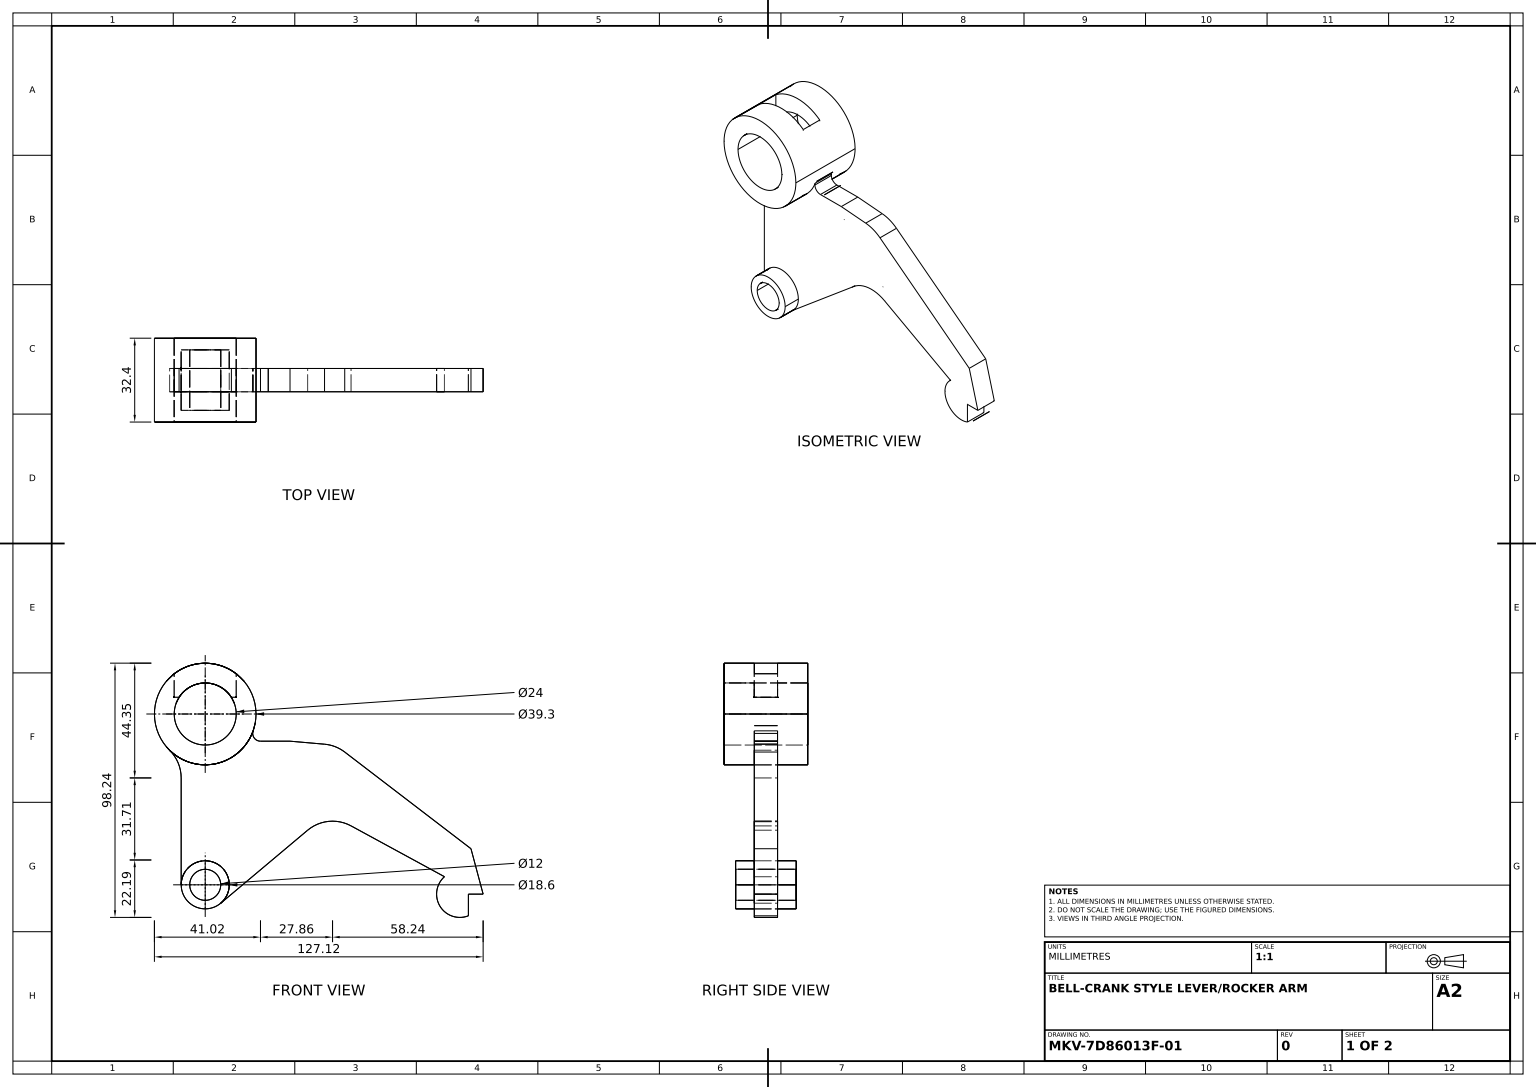
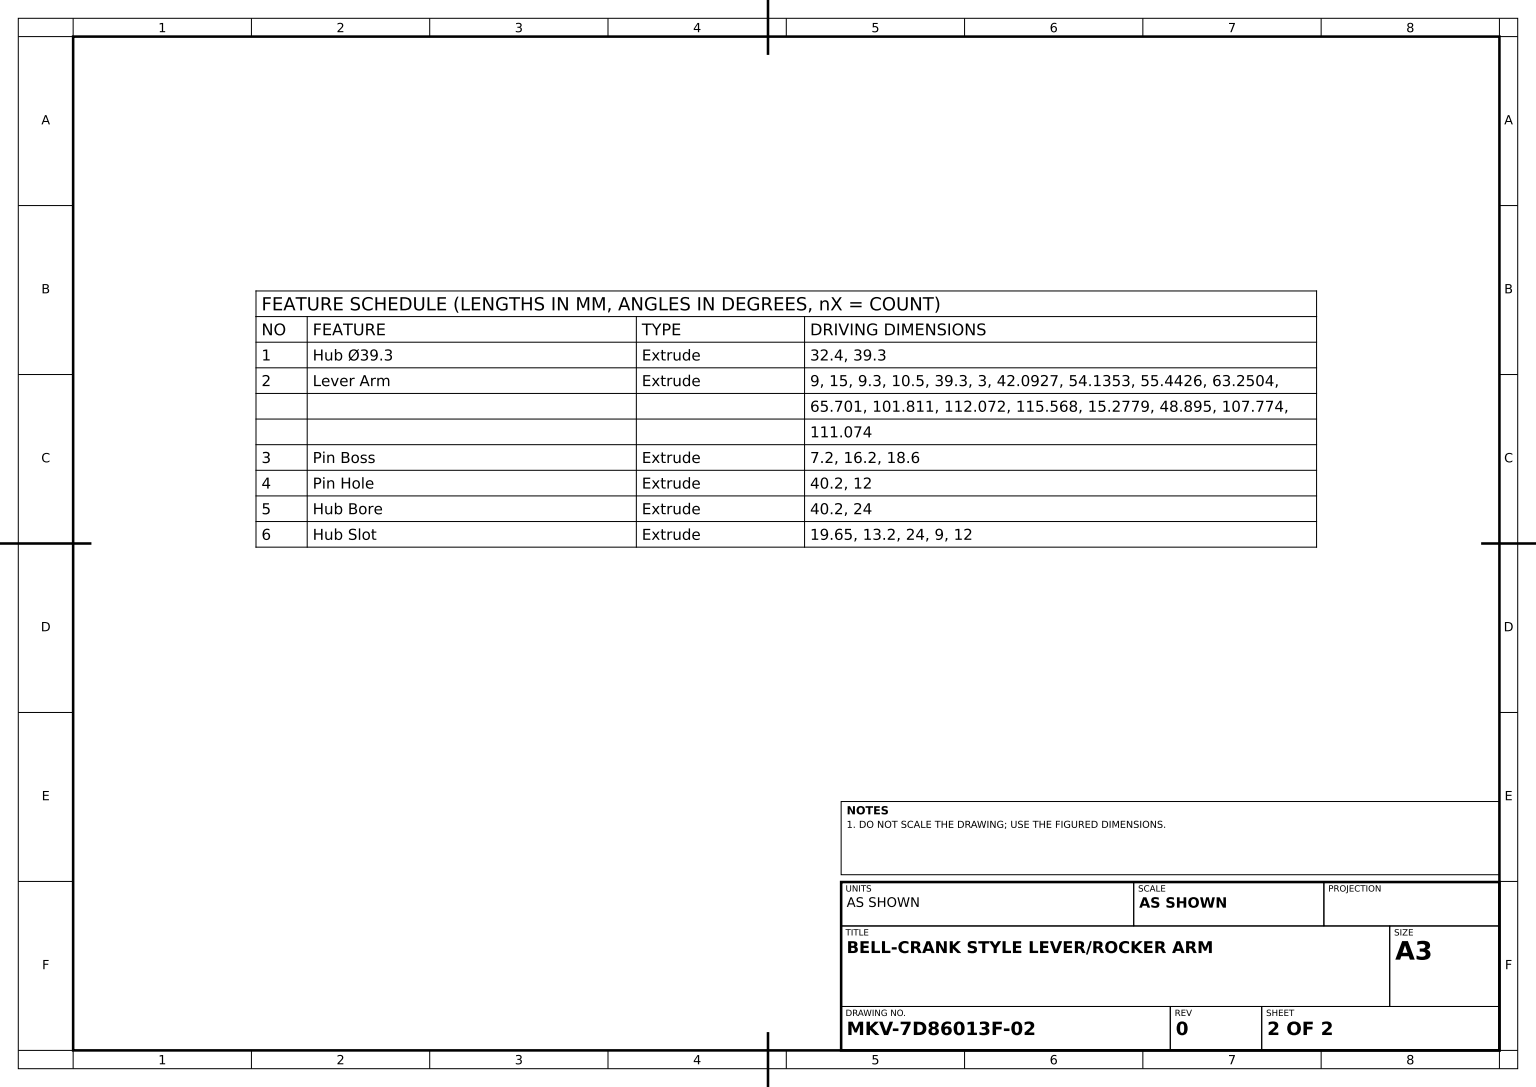
SolidWorks part; units mm, degrees
material "Plain Carbon Steel"
ref_plane "Front Plane" through (0, 0, 0) normal (0, 0, 1) x (1, 0, 0)
ref_plane "Top Plane" through (0, 0, 0) normal (0, 1, 0) x (1, 0, 0)
ref_plane "Right Plane" through (0, 0, 0) normal (1, 0, 0) x (0, 0, -1)
sketch "Hub Sketch" plane through (0, 0, 0) normal (0, 0, 1) x (1, 0, 0)
  circle A0 centre (0, 0) radius 19.65
  dimension "D1" = 39.3
extrude "Hub Ø39.3" add sketch "Hub Sketch" along normal mid plane 32.4
sketch "Lever Arm Sketch" plane through (0, 0, 0) normal (0, 0, 1) x (1, 0, 0)
  line L1 (-9.3, -66) -> (-9.3, -24.7009)
  line L4 (5.9779, -73.1242) -> (39.595, -44.9161)
  line L5 (21.3722, -10.5) -> (32.7927, -10.5)
  line L6 (56.401, -43.2282) -> (92.5111, -62.8585)
  line L7 (32.7927, -10.5) -> (46.1426, -11.668)
  line L8 (101.7737, -77.9732) -> (101.7737, -69.6)
  line L9 (101.7737, -69.6) -> (107.4737, -69.6)
  line L10 (107.4737, -69.6) -> (102.7724, -52.0545)
  line L11 (53.9504, -14.6981) -> (102.7724, -52.0545)
  arc A0 (-9.3, -66) -> (5.9779, -73.1242) centre (0, -66) ccw
  arc A3 (56.401, -43.2282) -> (39.595, -44.9161) centre (49.2368, -56.4068) ccw
  arc A4 (107.4737, -69.6) -> (106.2679, -65.1) centre (98.4737, -69.6) ccw
  arc A5 (92.5111, -62.8585) -> (101.7737, -77.9732) centre (98.4737, -69.6) ccw
  circle A6 centre (0, 0) radius 19.65
  arc A7 (46.1426, -11.668) -> (53.9504, -14.6981) centre (44.8353, -26.6109) cw
  arc A8 (-9.3, -24.7009) -> (-13.7805, -14.0078) centre (-24.3, -24.7009) ccw
  arc A9 (18.5415, -6.5066) -> (21.3722, -10.5) centre (21.3722, -7.5) ccw
  dimension "D1" = 15
  dimension "D5" = 39.3
  dimension "D6" = 3
  dimension "D2" = 9
  dimension "D3" = 9.3
  dimension "D4" = 10.5
  dimension "D7" = 15.2779
  dimension "D8" = 42.0927
  dimension "D9" = 48.895
  dimension "D10" = 54.1353
  dimension "D11" = 55.4426
  dimension "D12" = 107.7737
  dimension "D13" = 63.2504
  dimension "D14" = 65.701
  dimension "D15" = 101.8111
  dimension "D16" = 111.0737
  dimension "D18" = 112.0724
  dimension "D19" = 115.5679
extrude "Lever Arm" add sketch "Lever Arm Sketch" along normal mid plane 9 contours A9 A6 A8 L1 A0 L4 A3 L6 A5 L8 L9 L10 L11 A7 L7 L5
sketch "Pin Boss Sketch" plane through (0, 0, 4.5) normal (0, 0, 1) x (1, 0, 0)
  circle A0 centre (0, -66) radius 9.3
  dimension "D1" = 18.6
extrude "Pin Boss" add sketch "Pin Boss Sketch" along normal blind 7.2 and the other way blind 16.2
sketch "Pin Hole Sketch" plane through (0, 0, 11.7) normal (0, 0, 1) x (1, 0, 0)
  circle A0 centre (0, -66) radius 6
  dimension "D1" = 12
extrude "Pin Hole" cut sketch "Pin Hole Sketch" against normal blind 40.2
sketch "Hub Bore Sketch" plane through (0, 0, 16.2) normal (0, 0, 1) x (1, 0, 0)
  circle A0 centre (0, 0) radius 12
  dimension "D1" = 24
extrude "Hub Bore" cut sketch "Hub Bore Sketch" against normal blind 40.2
ref_plane "Hub Slot Plane" through (0, 19.65, 0) normal (0, 1, 0) x (1, 0, 0)
sketch "Hub Slot Sketch" plane through (0, 19.65, 0) normal (0, 1, 0) x (1, 0, 0)
  line L1 (-12, 0) -> (-12, 4.5)
  line L2 (-12, 4.5) -> (12, 4.5)
  line L3 (12, 4.5) -> (12, -4.5)
  line L4 (12, -4.5) -> (-12, -4.5)
  line L5 (-12, -4.5) -> (-12, 0)
  dimension "D1" = 24
  dimension "D2" = 9
  dimension "D3" = 12
extrude "Hub Slot" cut sketch "Hub Slot Sketch" against normal blind 13.2
